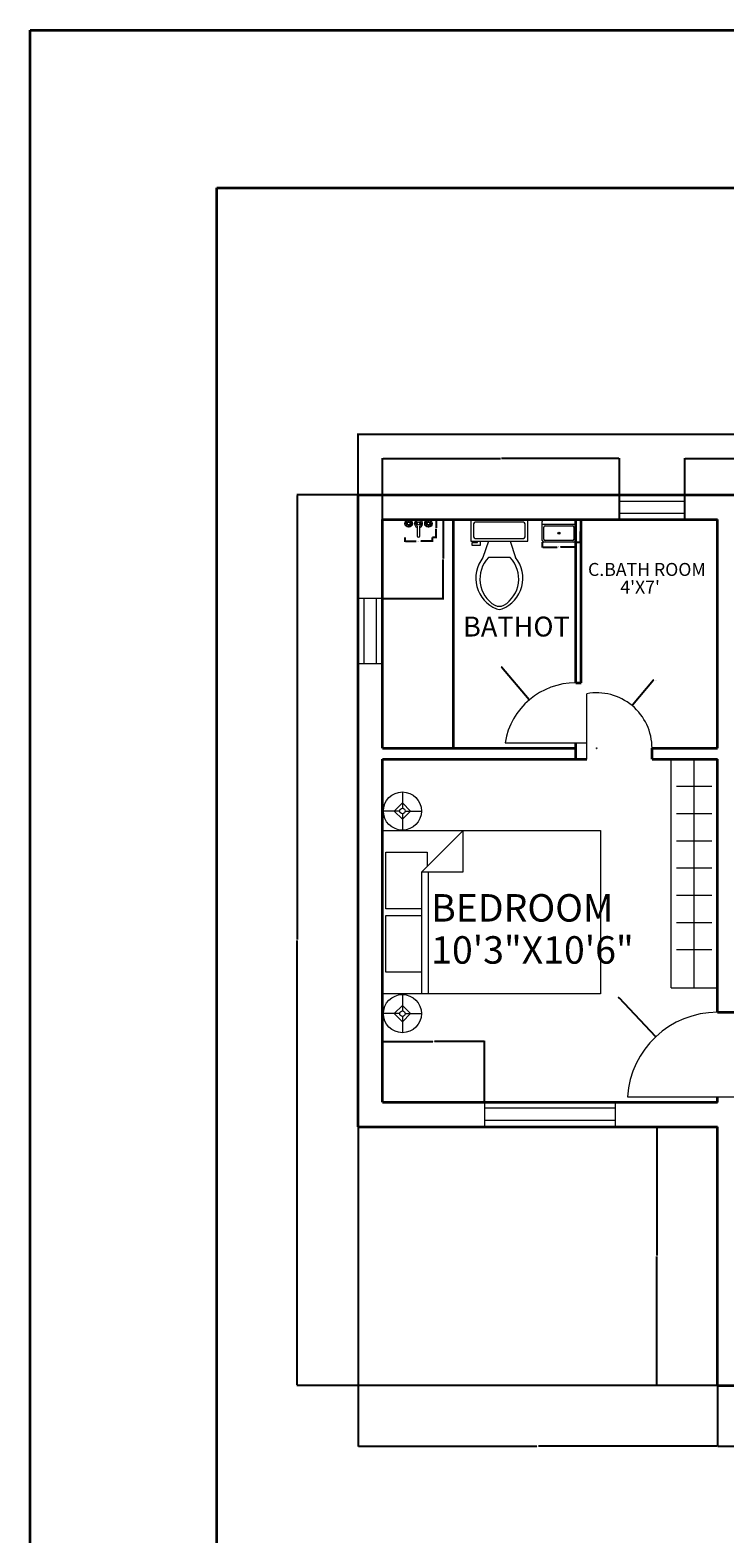
# Model space of a CAD drawing. Units: inches. Extents: x 2286 to 3750, y 1240 to 2345.
# Tile 4 of 7: x 2286 to 2541, y 1793 to 2345. Entities that reach past the tile are written whole.
import ezdxf

# ---------------------------------------------------------------- set-up
doc = ezdxf.new("R2010")
doc.units = ezdxf.units.IN
for name, color, linetype, lineweight in [('A-ANNO-DIMS', 2, 'Continuous', 18), ('A-AREA-IDEN', 7, 'Continuous', 18), ('A-DOOR', 4, 'Continuous', 18), ('A-FLOR-CASE', 8, 'Continuous', 18), ('A-FLOR-FIXT', 9, 'Continuous', 18), ('A-FURN', 8, 'Continuous', 18), ('A-GLAZ', 51, 'Continuous', 18), ('A-WALL', 7, 'Continuous', 35)]:
    doc.layers.add(name, color=color, linetype=linetype, lineweight=lineweight)
doc.styles.get("Standard").update_dxf_attribs({"font": 'arial.ttf'})
doc.dimstyles.get("Standard").update_dxf_attribs({"dimtxt": 0.18, "dimasz": 0.18, "dimexe": 0.18, "dimexo": 0.0625, "dimgap": 0.09, "dimtad": 0, "dimtih": 1, "dimtoh": 1, "dimdec": 4, "dimzin": 0, "dimdsep": 46, "dimtxsty": 'Standard', "dimcen": 0.09, "dimadec": 0, "dimazin": 0, "dimtfac": 1, "dimtdec": 4, "dimtofl": 0, "dimtmove": 0, "dimatfit": 3, "dimfxl": 1, "dimtolj": 1, "dimtzin": 0, "dimarcsym": 0})

# ---------------------------------------------------------------- blocks, each defined once
blk = doc.blocks.new('Toilet - top')
for p, q in [((9.5, -6), (9.5, -2)), ((-10, -8.5), (-8, -8.5)), ((-10, -9.5), (-10, -8.5)), ((-7, -9.5), (-10, -9.5)), ((-8, -8.5), (-8, -8)), ((-7, -8), (-7, -9.5)), ((-4, -8), (-6, -14)), ((4, -8), (6, -14)), ((4, -14), (-4, -14))]:
    blk.add_line(p, q)
blk.add_lwpolyline([(10.5, -8), (10.5, 0), (-10.5, 0), (-10.5, -8)], close=True)
for points in [[(-9.5, -2), (-9.5, -6)], [(8.5, -1), (-8.5, -1)], [(-8.5, -7), (8.5, -7)]]:
    blk.add_lwpolyline(points)
for centre, radius, start, end in [((-8.62, -1.88), 0.884, 81.8699, 188.1301), ((8.62, -1.88), 0.884, 351.8699, 98.1301), ((-8.62, -6.12), 0.884, 171.8699, 278.1301), ((8.62, -6.12), 0.884, 261.8699, 8.1301), ((3.52, -21.58), 12.17, 141.4691, 247.9714), ((4.2, -21.82), 11.33, 136.3677, 238.9468), ((-3.52, -21.58), 12.17, 292.0284, 38.5307), ((-4.2, -21.82), 11.33, 301.053, 43.6321), ((0, -27.88), 4, 245.7318, 294.2682), ((0, -29), 4, 254.8605, 285.1395)]:
    blk.add_arc(centre, radius, start, end)
blk = doc.blocks.new('Faucet - Bathroom top')
for p, q in [((-4.107, 0.125), (-4.375, 0.125)), ((-3.75, 0.4788), (-3.75, 0.75)), ((-3.5, 0.482), (-3.5, 0.75)), ((-3.1461, 0.125), (-2.875, 0.125)), ((3.143, 0.125), (2.875, 0.125)), ((3.5, 0.4788), (3.5, 0.75)), ((3.75, 0.482), (3.75, 0.75)), ((4.1039, 0.125), (4.375, 0.125)), ((-4.1039, -0.125), (-4.375, -0.125)), ((-3.75, -0.4821), (-3.75, -0.75)), ((-3.5, -0.4789), (-3.5, -0.75)), ((-3.143, -0.125), (-2.875, -0.125)), ((-0.5, -0.8639), (-0.5, -4.5)), ((0.5, -4.5), (0.5, -0.8631)), ((3.1461, -0.125), (2.875, -0.125)), ((3.5, -0.4821), (3.5, -0.75)), ((3.75, -0.4789), (3.75, -0.75)), ((4.107, -0.125), (4.375, -0.125))]:
    blk.add_line(p, q)
for centre, radius in [((-3.625, 0), 1.375), ((-4.625, 0), 0.2795), ((-3.625, 0), 0.5), ((-3.625, 1), 0.2795), ((-2.625, 0), 0.2795), ((0, 0), 0.5), ((3.625, 0), 1.375), ((2.625, 0), 0.2795), ((3.625, 0), 0.5), ((3.625, 1), 0.2795), ((4.625, 0), 0.2795), ((-3.625, -1), 0.2795), ((3.625, -1), 0.2795)]:
    blk.add_circle(centre, radius)
for centre, radius, start, end in [((-3.625, 0), 1, 105.2407, 164.2093), ((-3.625, 0), 1, 16.44125, 74.07887), ((0, 0), 1.5, 289.6514, 250.3603), ((0, 0), 1, 300.3431, 239.7554), ((3.625, 0), 1, 106.12, 164.0884), ((3.625, 0), 1, 16.23422, 73.90469), ((-3.625, 0), 1, 196.2342, 253.9047), ((-3.625, 0), 1, 286.12, 344.0884), ((0, -4.5), 0.5, 180, 0), ((3.625, 0), 1, 196.4413, 254.0789), ((3.625, 0), 1, 285.2407, 344.2093)]:
    blk.add_arc(centre, radius, start, end)
blk = doc.blocks.new('Bed - Queen')
for p, q in [((0, -80.00003), (0, 0)), ((0, 0), (59.99999, 0)), ((59.99999, 0), (59.99999, -80.00003)), ((7.99999, -1.2), (28.79998, -1.2)), ((7.99999, -14.4), (7.99999, -1.2)), ((28.79998, -1.2), (28.79998, -14.4)), ((31.19999, -1.2), (51.99999, -1.2)), ((31.19999, -14.4), (31.19999, -1.2)), ((51.99999, -1.2), (51.99999, -16.4)), ((0, -14.4), (44.8, -14.4)), ((59.99999, -29.6), (44.8, -14.4)), ((44.8, -14.4), (44.8, -29.6)), ((51.99999, -16.4), (46.79936, -16.4)), ((44.8, -16.8), (0, -16.8)), ((44.8, -29.6), (59.99999, -29.6)), ((59.99999, -80.00003), (0, -80.00003))]:
    blk.add_line(p, q)
blk = doc.blocks.new('Lamp - Table')
for p, q in [((0, 7), (0, 1)), ((-1, 0), (-7, 0)), ((0, 3), (-3, 0)), ((-3, 0), (0, -3)), ((3, 0), (0, 3)), ((0, -3), (3, 0)), ((1, 0), (7, 0)), ((0, -1), (0, -7))]:
    blk.add_line(p, q)
for radius in [7, 1]:
    blk.add_circle((0, 0), radius)
blk = doc.blocks.new('Sink-single - 30 in top')
blk.add_line((-15, -3.999996), (15, -3.999996))
for points in [[(-13.5, 0), (13.5, 0)], [(-15, -18.499996), (-15, -1.5)], [(-13.5, -17.499996), (-13.5, -6.499996)], [(-12.5, -5.499996), (12.5, -5.499996)], [(13.5, -6.499996), (13.5, -17.499996)], [(15, -1.5), (15, -18.499996)], [(13.5, -19.999996), (-13.5, -19.999996)], [(12.5, -18.499996), (-12.5, -18.499996)]]:
    blk.add_lwpolyline(points)
for radius in [1, 0.5]:
    blk.add_circle((0, -11.999996), radius)
for centre, radius, start, end in [((-13.5, -1.5), 1.5, 90, 180), ((-12.5, -6.499996), 1, 90, 180), ((12.5, -6.499996), 1, 0, 90), ((13.5, -1.5), 1.5, 0, 90), ((-13.5, -18.499996), 1.5, 180, 270), ((-12.5, -17.499996), 1, 180, 270), ((12.5, -17.499996), 1, 270, 0), ((13.5, -18.499996), 1.5, 270, 0)]:
    blk.add_arc(centre, radius, start, end)
blk = doc.blocks.new('WIN-48x9')
for p, q in [((0, 0), (0, 9)), ((0, 6.75), (48, 6.75)), ((48, 0), (48, 9)), ((0, 2.25), (48, 2.25))]:
    blk.add_line(p, q)
blk = doc.blocks.new('WIN-24x9')
for p, q in [((0, 0), (0, 9)), ((0, 6.75), (24, 6.75)), ((24, 0), (24, 9)), ((0, 2.25), (24, 2.25))]:
    blk.add_line(p, q)
blk = doc.blocks.new('CLOSET-RAIL-84')
for p, q in [((6.5, 0), (6.5, 84)), ((0, 74), (13, 74)), ((0, 64), (13, 64)), ((0, 54), (13, 54)), ((0, 44), (13, 44)), ((0, 34), (13, 34)), ((0, 24), (13, 24)), ((0, 14), (13, 14))]:
    blk.add_line(p, q)
blk = doc.blocks.new('*D50')
at = {"layer": 'A-ANNO-DIMS', "color": 0, "lineweight": -2, "transparency": 16777216}
for p, q in [((2423.9, 2158.6), (2423.9, 2156.98)), ((2424.08, 2157.16), (2428.03, 2157.16)), ((2433.72, 2157.16), (2429.76, 2157.16)), ((2433.9, 2158.6), (2433.9, 2156.98))]:
    blk.add_line(p, q, dxfattribs=at)
at = {"layer": 'A-ANNO-DIMS', "color": 0, "transparency": 16777216}
for points in [[(2424.08, 2157.19), (2424.08, 2157.13), (2423.9, 2157.16)], [(2433.72, 2157.19), (2433.72, 2157.13), (2433.9, 2157.16)]]:
    blk.add_solid(points, dxfattribs=at)
at = {"layer": 'Defpoints', "color": 0, "transparency": 16777216}
for p in [(2423.9, 2158.66), (2433.9, 2158.66), (2433.9, 2157.16)]:
    blk.add_point(p, dxfattribs=at)
at = {"layer": 'A-ANNO-DIMS', "color": 0, "transparency": 16777216, "insert": (2428.9, 2157.16), "char_height": 0.18, "attachment_point": 5}
blk.add_mtext('\\A1;BATH TAP 10', dxfattribs=at)
blk = doc.blocks.new('*D51')
at = {"layer": 'A-ANNO-DIMS', "color": 0, "lineweight": -2, "transparency": 16777216}
for p, q in [((2433.96, 2165.16), (2435.58, 2165.16)), ((2435.4, 2164.98), (2435.4, 2162.09)), ((2435.4, 2158.84), (2435.4, 2161.73)), ((2433.96, 2158.66), (2435.58, 2158.66))]:
    blk.add_line(p, q, dxfattribs=at)
at = {"layer": 'A-ANNO-DIMS', "color": 0, "transparency": 16777216}
for points in [[(2435.37, 2164.98), (2435.43, 2164.98), (2435.4, 2165.16)], [(2435.37, 2158.84), (2435.43, 2158.84), (2435.4, 2158.66)]]:
    blk.add_solid(points, dxfattribs=at)
at = {"layer": 'Defpoints', "color": 0, "transparency": 16777216}
for p in [(2433.9, 2165.16), (2435.4, 2165.16), (2433.9, 2158.66)]:
    blk.add_point(p, dxfattribs=at)
at = {"layer": 'A-ANNO-DIMS', "color": 0, "transparency": 16777216, "insert": (2435.4, 2161.91), "char_height": 0.18, "attachment_point": 5}
blk.add_mtext('\\A1;7', dxfattribs=at)
blk = doc.blocks.new('*D52')
at = {"layer": 'A-ANNO-DIMS', "color": 0, "lineweight": -2, "transparency": 16777216}
for p, q in [((2474.32, 2156.81), (2474.32, 2154.86)), ((2474.5, 2155.04), (2479.81, 2155.04)), ((2486.38, 2155.04), (2481.07, 2155.04)), ((2486.56, 2156.81), (2486.56, 2154.86))]:
    blk.add_line(p, q, dxfattribs=at)
at = {"layer": 'A-ANNO-DIMS', "color": 0, "transparency": 16777216}
for points in [[(2474.5, 2155.07), (2474.5, 2155.01), (2474.32, 2155.04)], [(2486.38, 2155.07), (2486.38, 2155.01), (2486.56, 2155.04)]]:
    blk.add_solid(points, dxfattribs=at)
at = {"layer": 'Defpoints', "color": 0, "transparency": 16777216}
for p in [(2474.32, 2156.88), (2486.56, 2156.88), (2486.56, 2155.04)]:
    blk.add_point(p, dxfattribs=at)
at = {"layer": 'A-ANNO-DIMS', "color": 0, "transparency": 16777216, "insert": (2480.44, 2155.04), "char_height": 0.18, "attachment_point": 5}
blk.add_mtext('\\A1;BASIN 12', dxfattribs=at)
blk = doc.blocks.new('*D53')
at = {"layer": 'A-ANNO-DIMS', "color": 0, "lineweight": -2, "transparency": 16777216}
for p, q in [((2486.62, 2165.03), (2488.58, 2165.03)), ((2488.4, 2164.85), (2488.4, 2161.14)), ((2488.4, 2157.06), (2488.4, 2160.77)), ((2486.62, 2156.88), (2488.58, 2156.88))]:
    blk.add_line(p, q, dxfattribs=at)
at = {"layer": 'A-ANNO-DIMS', "color": 0, "transparency": 16777216}
for points in [[(2488.37, 2164.85), (2488.43, 2164.85), (2488.4, 2165.03)], [(2488.37, 2157.06), (2488.43, 2157.06), (2488.4, 2156.88)]]:
    blk.add_solid(points, dxfattribs=at)
at = {"layer": 'Defpoints', "color": 0, "transparency": 16777216}
for p in [(2486.56, 2165.03), (2488.4, 2165.03), (2486.56, 2156.88)]:
    blk.add_point(p, dxfattribs=at)
at = {"layer": 'A-ANNO-DIMS', "color": 0, "transparency": 16777216, "insert": (2488.4, 2160.96), "char_height": 0.18, "attachment_point": 5}
blk.add_mtext('\\A1;8', dxfattribs=at)
blk = doc.blocks.new('*D58')
at = {"layer": 'A-ANNO-DIMS', "color": 0, "lineweight": -2, "transparency": 16777216}
for p, q in [((2406.66, 2174.25), (2406.66, 2196.67)), ((2406.84, 2196.49), (2623.37, 2196.49)), ((2840.48, 2196.49), (2623.96, 2196.49)), ((2840.66, 2174.25), (2840.66, 2196.67))]:
    blk.add_line(p, q, dxfattribs=at)
at = {"layer": 'A-ANNO-DIMS', "color": 0, "transparency": 16777216}
for points in [[(2406.84, 2196.52), (2406.84, 2196.46), (2406.66, 2196.49)], [(2840.48, 2196.52), (2840.48, 2196.46), (2840.66, 2196.49)]]:
    blk.add_solid(points, dxfattribs=at)
at = {"layer": 'Defpoints', "color": 0, "transparency": 16777216}
for p in [(2840.66, 2196.49), (2406.66, 2174.19), (2840.66, 2174.19)]:
    blk.add_point(p, dxfattribs=at)
at = {"layer": 'A-ANNO-DIMS', "color": 0, "transparency": 16777216, "insert": (2623.66, 2196.49), "char_height": 0.18, "attachment_point": 5}
blk.add_mtext('\\A1;434', dxfattribs=at)
blk = doc.blocks.new('*D59')
at = {"layer": 'A-ANNO-DIMS', "color": 0, "lineweight": -2, "transparency": 16777216}
for p, q in [((2406.6, 2174.19), (2384.18, 2174.19)), ((2384.36, 2174.01), (2384.36, 2010.87)), ((2384.36, 1847.37), (2384.36, 2010.51)), ((2538.6, 1847.19), (2384.18, 1847.19))]:
    blk.add_line(p, q, dxfattribs=at)
at = {"layer": 'A-ANNO-DIMS', "color": 0, "transparency": 16777216}
for points in [[(2384.33, 2174.01), (2384.39, 2174.01), (2384.36, 2174.19)], [(2384.33, 1847.37), (2384.39, 1847.37), (2384.36, 1847.19)]]:
    blk.add_solid(points, dxfattribs=at)
at = {"layer": 'Defpoints', "color": 0, "transparency": 16777216}
for p in [(2406.66, 2174.19), (2384.36, 1847.19), (2538.66, 1847.19)]:
    blk.add_point(p, dxfattribs=at)
at = {"layer": 'A-ANNO-DIMS', "color": 0, "transparency": 16777216, "insert": (2384.36, 2010.69), "char_height": 0.18, "attachment_point": 5}
blk.add_mtext('\\A1;327', dxfattribs=at)
blk = doc.blocks.new('*D60')
at = {"layer": 'A-ANNO-DIMS', "color": 0, "lineweight": -2, "transparency": 16777216}
for p, q in [((2406.66, 1942.13), (2406.66, 1824.71)), ((2538.66, 1942.13), (2538.66, 1824.71)), ((2406.84, 1824.89), (2472.38, 1824.89)), ((2538.48, 1824.89), (2472.94, 1824.89))]:
    blk.add_line(p, q, dxfattribs=at)
at = {"layer": 'A-ANNO-DIMS', "color": 0, "transparency": 16777216}
for points in [[(2406.84, 1824.92), (2406.84, 1824.86), (2406.66, 1824.89)], [(2538.48, 1824.92), (2538.48, 1824.86), (2538.66, 1824.89)]]:
    blk.add_solid(points, dxfattribs=at)
at = {"layer": 'Defpoints', "color": 0, "transparency": 16777216}
for p in [(2406.66, 1942.19), (2538.66, 1942.19), (2538.66, 1824.89)]:
    blk.add_point(p, dxfattribs=at)
at = {"layer": 'A-ANNO-DIMS', "color": 0, "transparency": 16777216, "insert": (2472.66, 1824.89), "char_height": 0.18, "attachment_point": 5}
blk.add_mtext('\\A1;132', dxfattribs=at)
blk = doc.blocks.new('*D61')
at = {"layer": 'A-ANNO-DIMS', "color": 0, "lineweight": -2, "transparency": 16777216}
for p, q in [((2538.66, 1847.13), (2538.66, 1824.71)), ((2810.66, 1847.13), (2810.66, 1824.71)), ((2538.84, 1824.89), (2674.37, 1824.89)), ((2810.48, 1824.89), (2674.95, 1824.89))]:
    blk.add_line(p, q, dxfattribs=at)
at = {"layer": 'A-ANNO-DIMS', "color": 0, "transparency": 16777216}
for points in [[(2538.84, 1824.92), (2538.84, 1824.86), (2538.66, 1824.89)], [(2810.48, 1824.92), (2810.48, 1824.86), (2810.66, 1824.89)]]:
    blk.add_solid(points, dxfattribs=at)
at = {"layer": 'Defpoints', "color": 0, "transparency": 16777216}
for p in [(2538.66, 1847.19), (2810.66, 1847.19), (2810.66, 1824.89)]:
    blk.add_point(p, dxfattribs=at)
at = {"layer": 'A-ANNO-DIMS', "color": 0, "transparency": 16777216, "insert": (2674.66, 1824.89), "char_height": 0.18, "attachment_point": 5}
blk.add_mtext('\\A1;272', dxfattribs=at)
blk = doc.blocks.new('*D63')
at = {"layer": 'A-ANNO-DIMS', "color": 0, "lineweight": -2, "transparency": 16777216}
for p, q in [((2538.6, 1942.19), (2516.18, 1942.19)), ((2516.36, 1942.01), (2516.36, 1894.87)), ((2516.36, 1847.37), (2516.36, 1894.51)), ((2538.6, 1847.19), (2516.18, 1847.19))]:
    blk.add_line(p, q, dxfattribs=at)
at = {"layer": 'A-ANNO-DIMS', "color": 0, "transparency": 16777216}
for points in [[(2516.33, 1942.01), (2516.39, 1942.01), (2516.36, 1942.19)], [(2516.33, 1847.37), (2516.39, 1847.37), (2516.36, 1847.19)]]:
    blk.add_solid(points, dxfattribs=at)
at = {"layer": 'Defpoints', "color": 0, "transparency": 16777216}
for p in [(2516.36, 1942.19), (2538.66, 1942.19), (2538.66, 1847.19)]:
    blk.add_point(p, dxfattribs=at)
at = {"layer": 'A-ANNO-DIMS', "color": 0, "transparency": 16777216, "insert": (2516.36, 1894.69), "char_height": 0.18, "attachment_point": 5}
blk.add_mtext('\\A1;95', dxfattribs=at)
blk = doc.blocks.new('*D66')
at = {"layer": 'A-ANNO-DIMS', "color": 0, "lineweight": -2, "transparency": 16777216}
for p, q in [((2415.66, 2165.25), (2415.66, 2187.67)), ((2415.84, 2187.49), (2458.94, 2187.49)), ((2502.48, 2187.49), (2459.38, 2187.49)), ((2502.66, 2165.25), (2502.66, 2187.67))]:
    blk.add_line(p, q, dxfattribs=at)
at = {"layer": 'A-ANNO-DIMS', "color": 0, "transparency": 16777216}
for points in [[(2415.84, 2187.52), (2415.84, 2187.46), (2415.66, 2187.49)], [(2502.48, 2187.52), (2502.48, 2187.46), (2502.66, 2187.49)]]:
    blk.add_solid(points, dxfattribs=at)
at = {"layer": 'Defpoints', "color": 0, "transparency": 16777216}
for p in [(2502.66, 2187.49), (2415.66, 2165.19), (2502.66, 2165.19)]:
    blk.add_point(p, dxfattribs=at)
at = {"layer": 'A-ANNO-DIMS', "color": 0, "transparency": 16777216, "insert": (2459.16, 2187.49), "char_height": 0.18, "attachment_point": 5}
blk.add_mtext('\\A1;87', dxfattribs=at)
blk = doc.blocks.new('*D67')
at = {"layer": 'A-ANNO-DIMS', "color": 0, "lineweight": -2, "transparency": 16777216}
for p, q in [((2526.66, 2165.25), (2526.66, 2187.67)), ((2526.84, 2187.49), (2597.53, 2187.49)), ((2668.98, 2187.49), (2598.3, 2187.49)), ((2669.16, 2165.25), (2669.16, 2187.67))]:
    blk.add_line(p, q, dxfattribs=at)
at = {"layer": 'A-ANNO-DIMS', "color": 0, "transparency": 16777216}
for points in [[(2526.84, 2187.52), (2526.84, 2187.46), (2526.66, 2187.49)], [(2668.98, 2187.52), (2668.98, 2187.46), (2669.16, 2187.49)]]:
    blk.add_solid(points, dxfattribs=at)
at = {"layer": 'Defpoints', "color": 0, "transparency": 16777216}
for p in [(2669.16, 2187.49), (2526.66, 2165.19), (2669.16, 2165.19)]:
    blk.add_point(p, dxfattribs=at)
at = {"layer": 'A-ANNO-DIMS', "color": 0, "transparency": 16777216, "insert": (2597.91, 2187.49), "char_height": 0.18, "attachment_point": 5}
blk.add_mtext('\\A1;142.5', dxfattribs=at)
blk = doc.blocks.new('*D68')
at = {"layer": 'A-ANNO-DIMS', "color": 0, "lineweight": -2, "transparency": 16777216}
for p, q in [((2415.73, 2165.19), (2438.14, 2165.19)), ((2437.96, 2165.01), (2437.96, 2150.87)), ((2437.96, 2136.37), (2437.96, 2150.51)), ((2415.73, 2136.19), (2438.14, 2136.19))]:
    blk.add_line(p, q, dxfattribs=at)
at = {"layer": 'A-ANNO-DIMS', "color": 0, "transparency": 16777216}
for points in [[(2437.93, 2165.01), (2437.99, 2165.01), (2437.96, 2165.19)], [(2437.93, 2136.37), (2437.99, 2136.37), (2437.96, 2136.19)]]:
    blk.add_solid(points, dxfattribs=at)
at = {"layer": 'Defpoints', "color": 0, "transparency": 16777216}
for p in [(2415.66, 2165.19), (2415.66, 2136.19), (2437.96, 2136.19)]:
    blk.add_point(p, dxfattribs=at)
at = {"layer": 'A-ANNO-DIMS', "color": 0, "transparency": 16777216, "insert": (2437.96, 2150.69), "char_height": 0.18, "attachment_point": 5}
blk.add_mtext('\\A1;29', dxfattribs=at)
blk = doc.blocks.new('*D69')
at = {"layer": 'A-ANNO-DIMS', "color": 0, "lineweight": -2, "transparency": 16777216}
for p, q in [((2415.66, 1951.25), (2415.66, 1973.67)), ((2415.84, 1973.49), (2434.09, 1973.49)), ((2452.98, 1973.49), (2434.74, 1973.49)), ((2453.16, 1951.25), (2453.16, 1973.67))]:
    blk.add_line(p, q, dxfattribs=at)
at = {"layer": 'A-ANNO-DIMS', "color": 0, "transparency": 16777216}
for points in [[(2415.84, 1973.52), (2415.84, 1973.46), (2415.66, 1973.49)], [(2452.98, 1973.52), (2452.98, 1973.46), (2453.16, 1973.49)]]:
    blk.add_solid(points, dxfattribs=at)
at = {"layer": 'Defpoints', "color": 0, "transparency": 16777216}
for p in [(2453.16, 1973.49), (2415.66, 1951.19), (2453.16, 1951.19)]:
    blk.add_point(p, dxfattribs=at)
at = {"layer": 'A-ANNO-DIMS', "color": 0, "transparency": 16777216, "insert": (2434.41, 1973.49), "char_height": 0.18, "attachment_point": 5}
blk.add_mtext('\\A1;37.5', dxfattribs=at)
blk = doc.blocks.new('*D124')
at = {"layer": 'A-ANNO-DIMS', "color": 0, "lineweight": -2, "transparency": 16777216}
for p, q in [((2502.26, 1989.68), (2502.44, 1989.68)), ((2502.44, 1989.68), (2515.9, 1975.35)), ((2538.57, 1951.12), (2538.75, 1951.12)), ((2538.66, 1951.03), (2538.66, 1951.21))]:
    blk.add_line(p, q, dxfattribs=at)
at = {"layer": 'A-ANNO-DIMS', "color": 0, "transparency": 16777216}
blk.add_solid([(2515.92, 1975.38), (2515.88, 1975.33), (2516.03, 1975.22)], dxfattribs=at)
at = {"layer": 'Defpoints', "color": 0, "transparency": 16777216}
for p in [(2516.03, 1975.22), (2538.66, 1951.12)]:
    blk.add_point(p, dxfattribs=at)
at = {"layer": 'A-ANNO-DIMS', "color": 0, "transparency": 16777216, "insert": (2501.71, 1989.68), "char_height": 0.18, "attachment_point": 5}
blk.add_mtext('\\A1;R33.065', dxfattribs=at)
blk = doc.blocks.new('*D126')
at = {"layer": 'A-ANNO-DIMS', "color": 0, "lineweight": -2, "transparency": 16777216}
for p, q in [((2459.24, 2111.03), (2459.42, 2111.03)), ((2459.42, 2111.03), (2469.52, 2099.09)), ((2486.57, 2078.83), (2486.75, 2078.83)), ((2486.66, 2078.74), (2486.66, 2078.92))]:
    blk.add_line(p, q, dxfattribs=at)
at = {"layer": 'A-ANNO-DIMS', "color": 0, "transparency": 16777216}
blk.add_solid([(2469.54, 2099.11), (2469.49, 2099.07), (2469.63, 2098.95)], dxfattribs=at)
at = {"layer": 'Defpoints', "color": 0, "transparency": 16777216}
for p in [(2469.63, 2098.95), (2486.66, 2078.83)]:
    blk.add_point(p, dxfattribs=at)
at = {"layer": 'A-ANNO-DIMS', "color": 0, "transparency": 16777216, "insert": (2458.69, 2111.03), "char_height": 0.18, "attachment_point": 5}
blk.add_mtext('\\A1;R26.364', dxfattribs=at)
blk = doc.blocks.new('*D127')
at = {"layer": 'A-ANNO-DIMS', "color": 0, "lineweight": -2, "transparency": 16777216}
for p, q in [((2515.16, 2106.18), (2507.46, 2096.95)), ((2515.34, 2106.18), (2515.16, 2106.18)), ((2494.24, 2081.19), (2494.42, 2081.19)), ((2494.33, 2081.1), (2494.33, 2081.28))]:
    blk.add_line(p, q, dxfattribs=at)
at = {"layer": 'A-ANNO-DIMS', "color": 0, "transparency": 16777216}
blk.add_solid([(2507.44, 2096.97), (2507.49, 2096.93), (2507.35, 2096.81)], dxfattribs=at)
at = {"layer": 'Defpoints', "color": 0, "transparency": 16777216}
for p in [(2507.35, 2096.81), (2494.33, 2081.19)]:
    blk.add_point(p, dxfattribs=at)
at = {"layer": 'A-ANNO-DIMS', "color": 0, "transparency": 16777216, "insert": (2515.89, 2106.18), "char_height": 0.18, "attachment_point": 5}
blk.add_mtext('\\A1;R20.333', dxfattribs=at)

msp = doc.modelspace()

# ---------------------------------------------------------------- linework, layer by layer
at = {"layer": 'A-DOOR'}
for p, q in [((2490.6637, 2077.1892), (2490.6637, 2101.1892)), ((2460.6637, 2083.1892), (2490.6637, 2083.1892)), ((2505.6637, 1953.1892), (2547.6637, 1953.1892))]:
    msp.add_line(p, q, dxfattribs=at)
for centre, radius, start, end in [((2486.6637, 2078.8256), 26.3636, 90, 170.472717), ((2494.3303, 2081.1892), 20.3333, 360, 100.388858), ((2538.6637, 1951.1247), 33.0645, 90, 176.420179)]:
    msp.add_arc(centre, radius, start, end, dxfattribs=at)
at = {"layer": 'A-FLOR-CASE'}
for q in [(2521.6637, 2077.1892), (2538.6637, 1993.1892)]:
    msp.add_line((2521.6637, 1993.1892), q, dxfattribs=at)
at = {"layer": 'A-WALL'}
for p, q in [((2406.6637, 2174.1892), (2840.6637, 2174.1892)), ((2406.6637, 1942.1892), (2406.6637, 2174.1892)), ((2415.6637, 2165.1892), (2538.6637, 2165.1892)), ((2415.6637, 2081.1892), (2415.6637, 2165.1892)), ((2441.6279, 2165.1892), (2441.6279, 2081.1892)), ((2486.6637, 2105.1892), (2486.6637, 2165.1892)), ((2488.6637, 2105.1892), (2488.6637, 2165.1892)), ((2538.6637, 2081.1892), (2538.6637, 2165.1892)), ((2486.6637, 2105.1892), (2488.6637, 2105.1892)), ((2486.6637, 2077.1892), (2486.6637, 2083.1892)), ((2415.6637, 2081.1892), (2486.6637, 2081.1892)), ((2415.6637, 2081.1892), (2486.6637, 2081.1892)), ((2415.6637, 1951.1892), (2415.6637, 2077.1892)), ((2415.6637, 2077.1892), (2490.6637, 2077.1892)), ((2514.6637, 2077.1892), (2514.6637, 2081.1892)), ((2514.6637, 2081.1892), (2538.6637, 2081.1892)), ((2514.6637, 2077.1892), (2538.6637, 2077.1892)), ((2538.6637, 1984.1892), (2538.6637, 2077.1892)), ((2538.6637, 1984.1892), (2544.6637, 1984.1892)), ((2415.6637, 1951.1892), (2538.6637, 1951.1892)), ((2538.6637, 1951.1892), (2538.6637, 1953.1892)), ((2406.6637, 1942.1892), (2538.6637, 1942.1892)), ((2538.6637, 1847.1892), (2538.6637, 1942.1892)), ((2538.6637, 1847.1892), (2810.6637, 1847.1892))]:
    msp.add_line(p, q, dxfattribs=at)
for points in [[(2286.2079, 2344.8717), (3750.2574, 2344.8717), (3750.2574, 1240.4105), (2286.2079, 1240.4105)], [(2354.794, 2286.8809), (3673.7575, 2286.8809), (3673.7575, 1335.3046), (2354.794, 1335.3046)]]:
    msp.add_lwpolyline(points, close=True, dxfattribs=at)

# ---------------------------------------------------------------- block references
at = {"layer": 'A-FLOR-CASE'}
msp.add_blockref('CLOSET-RAIL-84', (2523.6637, 1993.1892), dxfattribs=at)
at = {"layer": 'A-FLOR-FIXT'}
for name, p in [('Faucet - Bathroom top', (2428.8956, 2163.6642)), ('Toilet - top', (2458.5581, 2165.1601))]:
    msp.add_blockref(name, p, dxfattribs=at)
at = {"layer": 'A-FLOR-FIXT', "xscale": 0.4079720129753045, "yscale": 0.4079720129753045, "zscale": 0.4079720129753045}
msp.add_blockref('Sink-single - 30 in top', (2480.4403, 2165.0349), dxfattribs=at)
at = {"layer": 'A-FURN'}
for p in [(2422.9774, 2058.1031), (2422.9774, 1983.7032)]:
    msp.add_blockref('Lamp - Table', p, dxfattribs=at)
at = {"layer": 'A-FURN', "rotation": 90}
msp.add_blockref('Bed - Queen', (2415.6683, 1990.9454), dxfattribs=at)
at = {"layer": 'A-GLAZ'}
msp.add_blockref('WIN-24x9', (2502.6637, 2165.1892), dxfattribs=at)
for name, p, rotation in [('WIN-24x9', (2415.6637, 2112.1892), 89.99999999999856), ('WIN-48x9', (2501.1637, 1951.1892), 180)]:
    msp.add_blockref(name, p, dxfattribs=dict(at, rotation=rotation))

# ---------------------------------------------------------------- texts
at = {"layer": 'A-AREA-IDEN'}
for s, height, p in [('C.BATH ROOM', 4.756635, (2491.1479, 2144.434)), ("        4'X7'", 4.756635, (2491.3801, 2137.9649)), ('BATHOT', 7.30575, (2445.2361, 2122.183)), ('BEDROOM', 10.08366, (2433.5371, 2017.4972)), ('10\'3"X10\'6"', 10.083661, (2433.5371, 2002.0429))]:
    msp.add_text(s, height=height, dxfattribs=at).set_placement(p)

# ---------------------------------------------------------------- dimensions: what is measured, and where the dimension line sits
at = {"layer": 'A-ANNO-DIMS'}
for base, p1, p2, override, picture, middle in [((2840.6637, 2196.4892), (2406.6637, 2174.1892), (2840.6637, 2174.1892), {"dimdec": 0, "dimlfac": 1, "dimrnd": 0, "dimzin": 0, "dimdsep": 46, "dimlunit": 2}, '*D58', (2623.6637, 2196.4892)), ((2502.6637, 2187.4892), (2415.6637, 2165.1892), (2502.6637, 2165.1892), {"dimdec": 0, "dimlfac": 1, "dimrnd": 0, "dimzin": 0, "dimdsep": 46, "dimlunit": 2}, '*D66', (2459.1637, 2187.4892)), ((2453.1637, 1973.4892), (2415.6637, 1951.1892), (2453.1637, 1951.1892), {"dimdec": 1, "dimlfac": 1, "dimrnd": 0, "dimzin": 0, "dimdsep": 46, "dimlunit": 2}, '*D69', (2434.4137, 1973.4892)), ((2538.6637, 1824.8892), (2406.6637, 1942.1892), (2538.6637, 1942.1892), {"dimdec": 0, "dimlfac": 1, "dimrnd": 0, "dimzin": 0, "dimdsep": 46, "dimlunit": 2}, '*D60', (2472.6637, 1824.8892)), ((2810.6637, 1824.8892), (2538.6637, 1847.1892), (2810.6637, 1847.1892), {"dimdec": 0, "dimlfac": 1, "dimrnd": 0, "dimzin": 0, "dimdsep": 46, "dimlunit": 2}, '*D61', (2674.6637, 1824.8892))]:
    dim = msp.add_linear_dim(base=base, p1=p1, p2=p2, dimstyle='Standard', override=override, dxfattribs=at)
    dim.commit()
    dim.dimension.update_dxf_attribs({"geometry": picture, "text_midpoint": middle})
for base, p1, p2, angle, override, picture, middle in [((2669.1637, 2187.4892), (2526.6637, 2165.1892), (2669.1637, 2165.1892), 0, {"dimdec": 1, "dimlfac": 1, "dimrnd": 0, "dimzin": 0, "dimdsep": 46, "dimlunit": 2}, '*D67', (2597.9137, 2187.4892)), ((2384.3637, 1847.1892), (2406.6637, 2174.1892), (2538.6637, 1847.1892), 90, {"dimdec": 0, "dimlfac": 1, "dimrnd": 0, "dimzin": 0, "dimdsep": 46, "dimlunit": 2}, '*D59', (2384.3637, 2010.6892)), ((2437.9637, 2136.1892), (2415.6637, 2165.1892), (2415.6637, 2136.1892), 270, {"dimdec": 0, "dimlfac": 1, "dimrnd": 0, "dimzin": 0, "dimdsep": 46, "dimlunit": 2}, '*D68', (2437.9637, 2150.6892)), ((2435.39559, 2165.16424), (2433.89559, 2158.66416), (2433.89559, 2165.16424), 90, {"dimdec": 0, "dimlfac": 1, "dimrnd": 0, "dimzin": 0, "dimdsep": 46, "dimlunit": 2}, '*D51', (2435.39559, 2161.9142)), ((2488.3958, 2165.0349), (2486.5599, 2156.8755), (2486.5599, 2165.0349), 90, {"dimdec": 0, "dimlfac": 1, "dimrnd": 0, "dimzin": 0, "dimdsep": 46, "dimlunit": 2}, '*D53', (2488.3958, 2160.9552)), ((2516.3637, 1942.1892), (2538.6637, 1847.1892), (2538.6637, 1942.1892), 90, {"dimdec": 0, "dimlfac": 1, "dimrnd": 0, "dimzin": 0, "dimdsep": 46, "dimlunit": 2}, '*D63', (2516.3637, 1894.6892))]:
    dim = msp.add_linear_dim(base=base, p1=p1, p2=p2, angle=angle, dimstyle='Standard', override=override, dxfattribs=at)
    dim.commit()
    dim.dimension.update_dxf_attribs({"geometry": picture, "text_midpoint": middle})
for base, p1, p2, text, picture, middle in [((2433.8956, 2157.1642), (2423.8956, 2158.6642), (2433.8956, 2158.6642), 'BATH TAP <>', '*D50', (2428.8956, 2157.1642)), ((2486.5599, 2155.0396), (2474.3207, 2156.8755), (2486.5599, 2156.8755), 'BASIN <>', '*D52', (2480.4403, 2155.0396))]:
    dim = msp.add_linear_dim(base=base, p1=p1, p2=p2, text=text, dimstyle='Standard', override={"dimdec": 0, "dimlfac": 1, "dimrnd": 0, "dimzin": 0, "dimdsep": 46, "dimlunit": 2}, dxfattribs=at)
    dim.commit()
    dim.dimension.update_dxf_attribs({"geometry": picture, "text_midpoint": middle})
for center, mpoint, picture, middle in [((2486.6637, 2078.8256), (2469.634, 2098.951), '*D126', (2458.6868, 2111.0262)), ((2494.3303, 2081.1892), (2507.347, 2096.81), '*D127', (2515.8868, 2106.1825)), ((2538.66367, 1951.12467), (2516.02525, 1975.22373), '*D124', (2501.71177, 1989.68316))]:
    dim = msp.add_radius_dim(center=center, mpoint=mpoint, dimstyle='Standard', override={"dimdec": 3, "dimlfac": 1, "dimrnd": 0, "dimzin": 0, "dimdsep": 46, "dimlunit": 2}, dxfattribs=at)
    dim.commit()
    dim.dimension.update_dxf_attribs({"geometry": picture, "text_midpoint": middle, "dimtype": 164})

doc.saveas('drawing.dxf')
